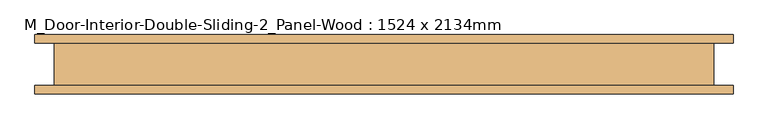
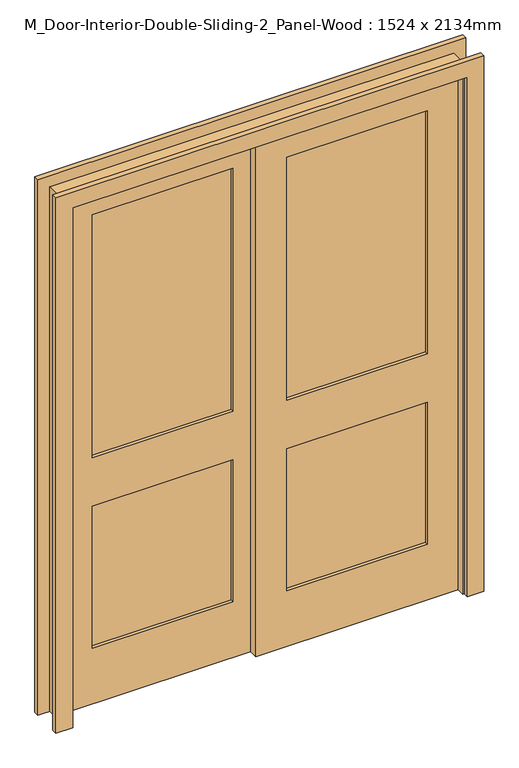
"""IFC4 building model written with IfcOpenShell, lengths in millimetres: door geometry, M_Door-Interior-Double-Sliding-2_Panel-Wood : 1524 x 2134mm."""

from ifc_helpers import new_model, si_unit, frame, origin, place, context, project, spatial, polyline, outline, extrude, source, transform, mapped, element, save


def m_door_interior_double_sliding_2_panel_wood_1524_x_2134mm_74d6d249(model_context):
    return source(origin(), model_context, "Body", "SweptSolid", [
        extrude(outline(polyline([(642.0, -10.7083333), (94.6, -10.7083333), (94.6, 0.9583333), (642.0, 0.9583333), (642.0, -10.7083333)])), frame((0.0, 0.0, 1014.4), z_axis=(0.0, 0.0, 1.0), x_axis=(1.0, 0.0, 0.0)), (0.0, 0.0, 1.0), 999.2),
        extrude(outline(polyline([(642.0, -10.7083333), (94.6, -10.7083333), (94.6, 0.9583333), (642.0, 0.9583333), (642.0, -10.7083333)])), frame((0.0, 0.0, 230.0), z_axis=(0.0, 0.0, 1.0), x_axis=(1.0, 0.0, 0.0)), (0.0, 0.0, 1.0), 584.4),
        extrude(outline(polyline([(2133.6, -25.4), (0.0, -25.4), (0.0, 762.0), (2133.6, 762.0), (2133.6, -25.4)]), holes=[polyline([(2013.6, 94.6), (2013.6, 642.0), (1014.4, 642.0), (1014.4, 94.6), (2013.6, 94.6)]), polyline([(814.4, 94.6), (814.4, 642.0), (230.0, 642.0), (230.0, 94.6), (814.4, 94.6)])]), frame((0.0, -22.375, 0.0), z_axis=(0.0, 1.0, 0.0), x_axis=(0.0, 0.0, 1.0)), (0.0, 0.0, 1.0), 35.0),
        extrude(outline(polyline([(-94.6, 24.2916667), (-642.0, 24.2916667), (-642.0, 35.9583333), (-94.6, 35.9583333), (-94.6, 24.2916667)])), frame((0.0, 0.0, 1014.4), z_axis=(0.0, 0.0, 1.0), x_axis=(1.0, 0.0, 0.0)), (0.0, 0.0, 1.0), 999.2),
        extrude(outline(polyline([(-94.6, 24.2916667), (-642.0, 24.2916667), (-642.0, 35.9583333), (-94.6, 35.9583333), (-94.6, 24.2916667)])), frame((0.0, 0.0, 230.0), z_axis=(0.0, 0.0, 1.0), x_axis=(1.0, 0.0, 0.0)), (0.0, 0.0, 1.0), 584.4),
        extrude(outline(polyline([(2133.6, -762.0), (0.0, -762.0), (0.0, 25.4), (2133.6, 25.4), (2133.6, -762.0)]), holes=[polyline([(2013.6, -642.0), (2013.6, -94.6), (1014.4, -94.6), (1014.4, -642.0), (2013.6, -642.0)]), polyline([(814.4, -642.0), (814.4, -94.6), (230.0, -94.6), (230.0, -642.0), (814.4, -642.0)])]), frame((0.0, 12.625, 0.0), z_axis=(0.0, 1.0, 0.0), x_axis=(0.0, 0.0, 1.0)), (0.0, 0.0, 1.0), 35.0),
        extrude(outline(polyline([(0.0, 762.0), (0.0, 787.0), (2158.6, 787.0), (2158.6, -787.0), (0.0, -787.0), (0.0, -762.0), (2133.6, -762.0), (2133.6, 762.0), (0.0, 762.0)])), frame((0.0, -53.975, 0.0), z_axis=(0.0, 1.0, 0.0), x_axis=(0.0, 0.0, 1.0)), (0.0, 0.0, 1.0), 101.6),
        extrude(outline(polyline([(0.0, 768.35), (0.0, 833.35), (2204.95, 833.35), (2204.95, -833.35), (0.0, -833.35), (0.0, -768.35), (2139.95, -768.35), (2139.95, 768.35), (0.0, 768.35)])), frame((0.0, -73.975, 0.0), z_axis=(0.0, 1.0, 0.0), x_axis=(0.0, 0.0, 1.0)), (0.0, 0.0, 1.0), 20.0),
        extrude(outline(polyline([(0.0, 768.35), (0.0, 833.35), (2204.95, 833.35), (2204.95, -833.35), (0.0, -833.35), (0.0, -768.35), (2139.95, -768.35), (2139.95, 768.35), (0.0, 768.35)])), frame((0.0, 47.625, 0.0), z_axis=(0.0, 1.0, 0.0), x_axis=(0.0, 0.0, 1.0)), (0.0, 0.0, 1.0), 20.0),
    ])


if __name__ == "__main__":
    model = new_model("IFC4")
    model_context = context("Model", 3, world=origin())
    ifc_project = project(units=[si_unit("LENGTHUNIT", "METRE", prefix="MILLI")], contexts=[model_context])
    site = spatial("IfcSite", under=ifc_project)
    building = spatial("IfcBuilding", under=site)
    placement = place(None, origin())
    m_door_interior_double_sliding_2_panel_wood_1524_x_2134mm_shape = m_door_interior_double_sliding_2_panel_wood_1524_x_2134mm_74d6d249(model_context)
    element("IfcDoor", 1, ObjectType="M_Door-Interior-Double-Sliding-2_Panel-Wood : 1524 x 2134mm", at=placement, inside=building, context=model_context, shape_type="MappedRepresentation", body=[
        mapped(m_door_interior_double_sliding_2_panel_wood_1524_x_2134mm_shape, transform((0.0, 0.0, 0.0), x_axis=(1.0, 0.0, 0.0), y_axis=(0.0, 1.0, 0.0), z_axis=(0.0, 0.0, 1.0))),
    ])
    save(model, "model.ifc")

# Revit data of these elements
# Type "M_Door-Interior-Double-Sliding-2_Panel-Wood : 1524 x 2134mm"
#   Type Mark = "9"
#   Assembly Code = "C1020300"
#   Analytic Construction = "Wooden"
#   Top Rail = 0' - 4.72441"
#   Thickness = 0' - 1.37795"
#   Thermal Resistance (R) = 2.5876 (h·ft²·°F)/BTU
#   Stiles = 0' - 4.72441"
#   Rough Width = 5' - 1.9685"
#   Rough Height = 7' - 0.98425"
#   Lock Rail = 0' - 7.87402"
#   Height = 7' - 0"
#   Width = 5' - 0"
#   Heat Transfer Coefficient (U) = 0.3865 BTU/(h·ft²·°F)
#   Bottom Rail = 0' - 9.05512"
#   Trim Material = Cherry
#   Panel Material = Cherry
#   Frame Material = Cherry
#   Visual Light Transmittance = 0
#   Solar Heat Gain Coefficient = 0
#   Wall Closure = (empty or 0)
#   Function = (empty or 0)
# Element 1 (IfcDoor, "M_Door-Interior-Double-Sliding-2_Panel-Wood : 1524 x 2134mm")
#   Materials on its faces: "Cherry"
# Materials
#   "Cherry": class "Wood", colour RGB 226 177 128, transparency 0, Description = "Prunus Serotina", Cost = 0
